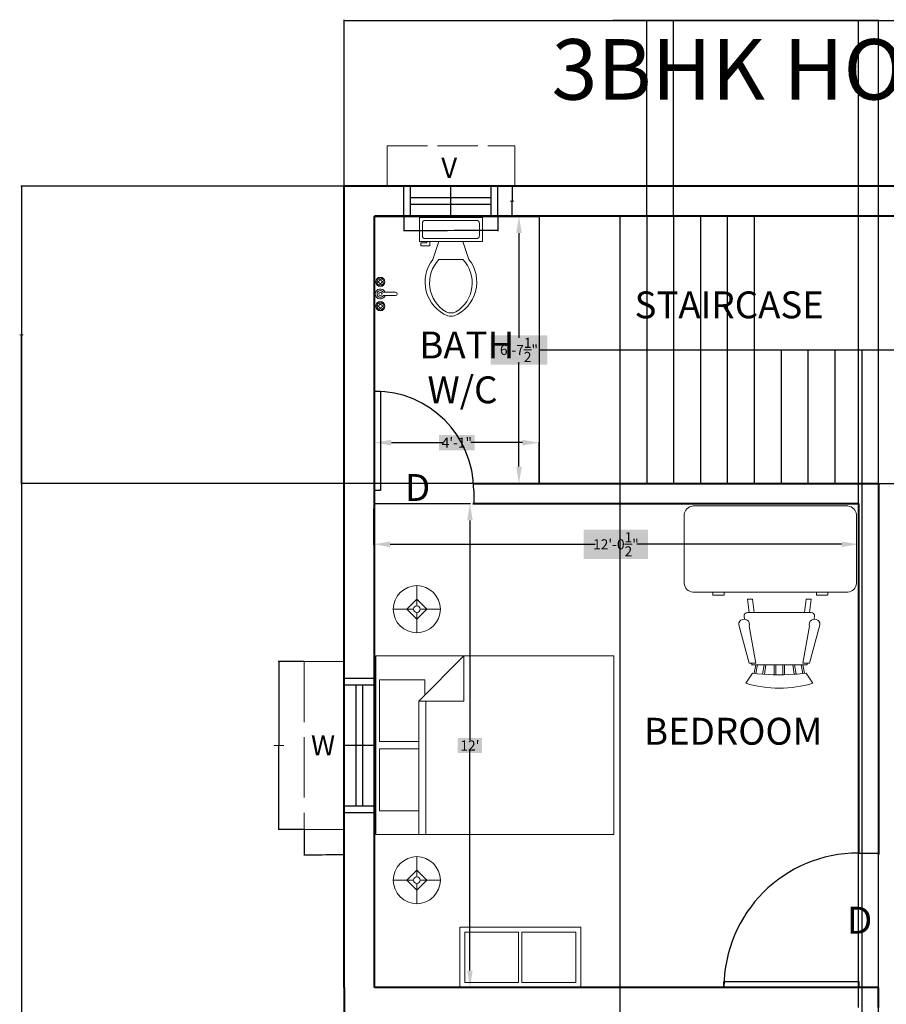
# Model space of a CAD drawing. Units: inches. Extents: x -301 to 715, y -607 to 364.
# Tile 104 of 141: x -301 to -43, y 67 to 360. Entities that reach past the tile are written whole.
import ezdxf

# ---------------------------------------------------------------- set-up
doc = ezdxf.new("R2010")
doc.units = ezdxf.units.IN
doc.header["$MEASUREMENT"] = 0
doc.linetypes.add('ACAD_ISO02W100', pattern=[15, 12, -3])
for name, color, linetype, lineweight in [('A-ANNO-DIMS', 2, 'Continuous', 18), ('A-ANNO-TEXT', 4, 'Continuous', 18), ('A-ANNO-TITL', 1, 'Continuous', 35), ('A-AREA-IDEN', 220, 'Continuous', 25), ('A-DOOR', 4, 'Continuous', 25), ('A-FLOR-CASE', 8, 'Continuous', 18), ('A-FLOR-FIXT', 9, 'Continuous', 18), ('A-FLOR-STRS', 2, 'Continuous', 25), ('A-FURN', 8, 'Continuous', 18), ('A-GLAZ', 2, 'Continuous', 25), ('A-GLAZ-OVHD', 2, 'ACAD_ISO02W100', 18), ('A-WALL', 3, 'Continuous', 40)]:
    doc.layers.add(name, color=color, linetype=linetype, lineweight=lineweight)
doc.styles.get("Standard").update_dxf_attribs({"font": 'arial.ttf'})
doc.dimstyles.get("Standard").update_dxf_attribs({"dimtxt": 0.18, "dimasz": 0.18, "dimexe": 0.18, "dimexo": 0.0625, "dimgap": 0.09, "dimtad": 0, "dimtih": 1, "dimtoh": 1, "dimdec": 1, "dimzin": 0, "dimdsep": 46, "dimlunit": 4, "dimtxsty": 'Standard', "dimcen": 0.09, "dimclrd": 3, "dimclre": 4, "dimclrt": 6, "dimadec": 0, "dimazin": 0, "dimtfac": 1, "dimtdec": 1, "dimtofl": 0, "dimtmove": 0, "dimatfit": 3, "dimfxl": 1, "dimtfill": 2, "dimtfillclr": 51, "dimtolj": 1, "dimtzin": 0, "dimarcsym": 0})

# ---------------------------------------------------------------- blocks, each defined once
blk = doc.blocks.new('*U4')
for p, q in [((0, 0), (0, -6)), ((40, 0), (40, -6))]:
    blk.add_line(p, q)
blk.add_lwpolyline([(0, 0), (0, 40), (1.75, 40), (1.75, 0)], close=True)
blk.add_arc((0, 0), 40, 0, 90)
blk = doc.blocks.new('Bed - Queen')
for p, q in [((0, -80.00003), (0, 0)), ((0, 0), (59.99999, 0)), ((59.99999, 0), (59.99999, -80.00003)), ((7.99999, -1.2), (28.79998, -1.2)), ((7.99999, -14.4), (7.99999, -1.2)), ((28.79998, -1.2), (28.79998, -14.4)), ((31.19999, -1.2), (51.99999, -1.2)), ((31.19999, -14.4), (31.19999, -1.2)), ((51.99999, -1.2), (51.99999, -16.4)), ((0, -14.4), (44.8, -14.4)), ((59.99999, -29.6), (44.8, -14.4)), ((44.8, -14.4), (44.8, -29.6)), ((51.99999, -16.4), (46.79936, -16.4)), ((44.8, -16.8), (0, -16.8)), ((44.8, -29.6), (59.99999, -29.6)), ((59.99999, -80.00003), (0, -80.00003))]:
    blk.add_line(p, q)
blk = doc.blocks.new('Lamp - Table')
for p, q in [((0, 7), (0, 1)), ((0, 3), (-3, 0)), ((3, 0), (0, 3)), ((-1, 0), (-7, 0)), ((-3, 0), (0, -3)), ((0, -3), (3, 0)), ((1, 0), (7, 0)), ((0, -1), (0, -7))]:
    blk.add_line(p, q)
for radius in [7, 1]:
    blk.add_circle((0, 0), radius)
blk = doc.blocks.new('Desk - 30 x 60 in.')
for p, q in [((-26.999995, 0), (26.999995, 0)), ((-29.999995, -27), (-29.999995, -3)), ((29.999995, -3), (29.999995, -27)), ((26.999995, -30), (-26.999995, -30)), ((-20.000005, -30), (-20.000005, -31)), ((-16.000005, -31), (-16.000005, -30)), ((15.999995, -31), (15.999995, -30)), ((19.999995, -30), (19.999995, -31)), ((-20.000005, -31), (-16.000005, -31)), ((19.999995, -31), (15.999995, -31))]:
    blk.add_line(p, q)
for centre, start, end in [((-26.499995, -3.5), 98.1301, 171.8699), ((26.499995, -3.5), 8.130102, 81.8699), ((-26.499995, -26.5), 188.1301, 261.8699), ((26.499995, -26.5), 278.1301, 351.8699)]:
    blk.add_arc(centre, 3.535534, start, end)
blk = doc.blocks.new('Chair - Rocking')
for p, q in [((-8, -4.5), (-10, -1.5)), ((8, -4.5), (10, -1.5)), ((-7.5, -4.5), (-7, -7)), ((-6.5, -7), (-7.02225, -4.43)), ((-4.5, -7), (-4.96674, -4.19951)), ((-4, -7), (-4.40532, -4.16272)), ((-1.5, -4.05012), (-1.5, -7)), ((-1, -7), (-1, -4.05012)), ((1, -7), (1, -4.04655)), ((1.5, -4.05012), (1.5, -7)), ((4, -7), (4.40187, -4.18694)), ((4.5, -7), (4.96761, -4.19437)), ((6.5, -7), (7, -4.4057)), ((7.5, -4.5), (7, -7)), ((-9, -7.5), (-12, -18.49999)), ((-7, -7.5), (-9, -7.5)), ((-9, -18.49999), (-7, -7.5)), ((-8.23428, -6.99939), (-8.3093, -7.47958)), ((-8.23041, -7), (8.23915, -7)), ((7, -7.5), (9, -7.5)), ((9, -18.49999), (7, -7.5)), ((8.31071, -7.48854), (8.23449, -7.00073)), ((9, -7.5), (12, -18.49999)), ((-10.36644, -20.64523), (-10.5, -21.49999)), ((-9, -22.49999), (-9.5, -26.49999)), ((0, -22.49999), (-9.5, -22.49999)), ((-8, -26.49999), (-7.5, -22.49999)), ((0, -22.49999), (9.5, -22.49999)), ((8, -26.49999), (7.5, -22.49999)), ((9, -22.49999), (9.5, -26.49999)), ((10.5, -21.49999), (10.3575, -20.58798)), ((-9.5, -26.49999), (-8, -26.49999)), ((9.5, -26.49999), (8, -26.49999))]:
    blk.add_line(p, q)
for centre, radius, start, end in [((0, -34.08333), 34.08333, 72.93847, 107.0615), ((0, -68.25004), 64.25, 93.92211, 97.15267), ((0, -68.25004), 64.25, 82.84733, 93.92211), ((-10.5, -18.99999), 1.58114, 161.5651, 18.43495), ((10.5, -18.99999), 1.58114, 161.5651, 18.43495), ((-9.5, -21.49999), 1, 180, 270), ((9.5, -21.49999), 1, 270, 0)]:
    blk.add_arc(centre, radius, start, end)
blk = doc.blocks.new('Wall Cabinet - 18 x 36 in front')
for p, q in [((17.5, -1.5), (17.5, -16.5)), ((18.5, -16.5), (18.5, -1.5))]:
    blk.add_line(p, q)
blk.add_lwpolyline([(0, -18), (0, 0), (36, 0), (36, -18)], close=True)
for points in [[(17.5, -16.5), (1.5, -16.5), (1.5, -1.5), (17.5, -1.5)], [(18.5, -1.5), (34.5, -1.5), (34.5, -16.5), (18.5, -16.5)]]:
    blk.add_lwpolyline(points)
blk = doc.blocks.new('*U2')
for p, q in [((0, 0), (0, -100)), ((750, 0), (750, -100))]:
    blk.add_line(p, q)
blk.add_lwpolyline([(0, 0), (0, 750), (43.75, 750), (43.75, 0)], close=True)
blk.add_arc((0, 0), 750, 0, 90)
blk = doc.blocks.new('Toilet - top')
for p, q in [((9.5, -6), (9.5, -2)), ((-10, -8.5), (-8, -8.5)), ((-10, -9.5), (-10, -8.5)), ((-7, -9.5), (-10, -9.5)), ((-8, -8.5), (-8, -8)), ((-7, -8), (-7, -9.5)), ((-4, -8), (-6, -14)), ((4, -8), (6, -14)), ((4, -14), (-4, -14))]:
    blk.add_line(p, q)
blk.add_lwpolyline([(10.5, -8), (10.5, 0), (-10.5, 0), (-10.5, -8)], close=True)
for points in [[(-9.5, -2), (-9.5, -6)], [(8.5, -1), (-8.5, -1)], [(-8.5, -7), (8.5, -7)]]:
    blk.add_lwpolyline(points)
for centre, radius, start, end in [((-8.62, -1.88), 0.884, 81.8699, 188.1301), ((8.62, -1.88), 0.884, 351.8699, 98.1301), ((-8.62, -6.12), 0.884, 171.8699, 278.1301), ((8.62, -6.12), 0.884, 261.8699, 8.1301), ((3.52, -21.58), 12.17, 141.4691, 247.9714), ((4.2, -21.82), 11.33, 136.3677, 238.9468), ((-3.52, -21.58), 12.17, 292.0284, 38.5307), ((-4.2, -21.82), 11.33, 301.053, 43.6321), ((0, -27.88), 4, 245.7318, 294.2682), ((0, -29), 4, 254.8605, 285.1395)]:
    blk.add_arc(centre, radius, start, end)
blk = doc.blocks.new('Faucet - Bathroom top')
for p, q in [((-4.107, 0.125), (-4.375, 0.125)), ((-3.75, 0.4788), (-3.75, 0.75)), ((-3.5, 0.482), (-3.5, 0.75)), ((-3.1461, 0.125), (-2.875, 0.125)), ((3.143, 0.125), (2.875, 0.125)), ((3.5, 0.4788), (3.5, 0.75)), ((3.75, 0.482), (3.75, 0.75)), ((4.1039, 0.125), (4.375, 0.125)), ((-4.1039, -0.125), (-4.375, -0.125)), ((-3.75, -0.4821), (-3.75, -0.75)), ((-3.5, -0.4789), (-3.5, -0.75)), ((-3.143, -0.125), (-2.875, -0.125)), ((-0.5, -0.8639), (-0.5, -4.5)), ((0.5, -4.5), (0.5, -0.8631)), ((3.1461, -0.125), (2.875, -0.125)), ((3.5, -0.4821), (3.5, -0.75)), ((3.75, -0.4789), (3.75, -0.75)), ((4.107, -0.125), (4.375, -0.125))]:
    blk.add_line(p, q)
for centre, radius in [((-3.625, 0), 1.375), ((-4.625, 0), 0.2795), ((-3.625, 0), 0.5), ((-3.625, 1), 0.2795), ((-2.625, 0), 0.2795), ((0, 0), 0.5), ((3.625, 0), 1.375), ((2.625, 0), 0.2795), ((3.625, 0), 0.5), ((3.625, 1), 0.2795), ((4.625, 0), 0.2795), ((-3.625, -1), 0.2795), ((3.625, -1), 0.2795)]:
    blk.add_circle(centre, radius)
for centre, radius, start, end in [((-3.625, 0), 1, 105.2407, 164.2093), ((-3.625, 0), 1, 16.44125, 74.07887), ((0, 0), 1.5, 289.6514, 250.3603), ((0, 0), 1, 300.3431, 239.7554), ((3.625, 0), 1, 106.12, 164.0884), ((3.625, 0), 1, 16.23422, 73.90469), ((-3.625, 0), 1, 196.2342, 253.9047), ((-3.625, 0), 1, 286.12, 344.0884), ((3.625, 0), 1, 196.4413, 254.0789), ((3.625, 0), 1, 285.2407, 344.2093), ((0, -4.5), 0.5, 180, 0)]:
    blk.add_arc(centre, radius, start, end)
blk = doc.blocks.new('*D52')
at = {"layer": 'A-ANNO-DIMS', "color": 0, "lineweight": -2, "transparency": 16777216}
for p, q in [((-195.6, 224.09), (-195.6, 234.01)), ((-190.6, 233.83), (-175.24, 233.83)), ((-151.6, 233.83), (-166.97, 233.83)), ((-146.6, 221.74), (-146.6, 234.01))]:
    blk.add_line(p, q, dxfattribs=at)
at = {"layer": 'A-ANNO-DIMS', "color": 0, "transparency": 16777216}
for points in [[(-190.6, 234.66), (-190.6, 232.99), (-195.6, 233.83)], [(-151.6, 234.66), (-151.6, 232.99), (-146.6, 233.83)]]:
    blk.add_solid(points, dxfattribs=at)
at = {"layer": 'Defpoints', "color": 0, "transparency": 16777216}
for p in [(-195.6, 233.83), (-195.6, 224.03), (-146.6, 221.68)]:
    blk.add_point(p, dxfattribs=at)
at = {"layer": 'A-ANNO-DIMS', "color": 0, "transparency": 16777216, "insert": (-171.1, 233.83), "char_height": 3, "attachment_point": 5, "bg_fill": 1, "box_fill_scale": 1.25, "bg_fill_color": 51, "bg_fill_transparency": 0}
blk.add_mtext('\\A1;4\'-1"', dxfattribs=at)
blk = doc.blocks.new('*D53')
at = {"layer": 'A-ANNO-DIMS', "color": 0, "lineweight": -2, "transparency": 16777216}
for p, q in [((-146.67, 301.18), (-152.79, 301.18)), ((-146.67, 221.68), (-152.79, 221.68))]:
    blk.add_line(p, q, dxfattribs=at)
at = {"layer": 'A-ANNO-DIMS', "color": 0, "lineweight": 30, "transparency": 16777216}
for p, q in [((-152.61, 296.18), (-152.61, 265.06)), ((-152.61, 226.68), (-152.61, 257.8))]:
    blk.add_line(p, q, dxfattribs=at)
at = {"layer": 'A-ANNO-DIMS', "color": 0, "transparency": 16777216}
for points in [[(-153.45, 296.18), (-151.78, 296.18), (-152.61, 301.18)], [(-153.45, 226.68), (-151.78, 226.68), (-152.61, 221.68)]]:
    blk.add_solid(points, dxfattribs=at)
at = {"layer": 'Defpoints', "color": 0, "transparency": 16777216}
for p in [(-146.6, 301.18), (-152.61, 221.68), (-146.6, 221.68)]:
    blk.add_point(p, dxfattribs=at)
at = {"layer": 'A-ANNO-DIMS', "color": 0, "transparency": 16777216, "insert": (-152.61, 261.43), "char_height": 3, "attachment_point": 5, "bg_fill": 1, "box_fill_scale": 1.25, "bg_fill_color": 51, "bg_fill_transparency": 0}
blk.add_mtext('\\A1;6\'-7{\\H1x;\\S1/2;}"', dxfattribs=at)
blk = doc.blocks.new('*D54')
at = {"layer": 'A-ANNO-DIMS', "color": 0, "lineweight": -2, "transparency": 16777216}
for p, q in [((-195.92, 214.14), (-195.92, 203.39)), ((-51.6, 215.62), (-51.6, 203.39)), ((-190.92, 203.57), (-129.96, 203.57)), ((-56.6, 203.57), (-117.57, 203.57))]:
    blk.add_line(p, q, dxfattribs=at)
at = {"layer": 'A-ANNO-DIMS', "color": 0, "transparency": 16777216}
for points in [[(-190.92, 204.4), (-190.92, 202.73), (-195.92, 203.57)], [(-56.6, 204.4), (-56.6, 202.73), (-51.6, 203.57)]]:
    blk.add_solid(points, dxfattribs=at)
at = {"layer": 'Defpoints', "color": 0, "transparency": 16777216}
for p in [(-195.92, 214.2), (-51.6, 215.68), (-195.92, 203.57)]:
    blk.add_point(p, dxfattribs=at)
at = {"layer": 'A-ANNO-DIMS', "color": 0, "transparency": 16777216, "insert": (-123.76, 203.57), "char_height": 3, "attachment_point": 5, "bg_fill": 1, "box_fill_scale": 1.25, "bg_fill_color": 51, "bg_fill_transparency": 0}
blk.add_mtext('\\A1;12\'-0{\\H1x;\\S1/2;}"', dxfattribs=at)
blk = doc.blocks.new('*D55')
at = {"layer": 'A-ANNO-DIMS', "color": 0, "lineweight": -2, "transparency": 16777216}
for p, q in [((-195.54, 215.68), (-167.03, 215.68)), ((-167.21, 210.68), (-167.21, 145.28)), ((-167.21, 76.68), (-167.21, 142.09)), ((-195.54, 71.68), (-167.03, 71.68))]:
    blk.add_line(p, q, dxfattribs=at)
at = {"layer": 'A-ANNO-DIMS', "color": 0, "transparency": 16777216}
for points in [[(-168.04, 210.68), (-166.38, 210.68), (-167.21, 215.68)], [(-168.04, 76.68), (-166.38, 76.68), (-167.21, 71.68)]]:
    blk.add_solid(points, dxfattribs=at)
at = {"layer": 'Defpoints', "color": 0, "transparency": 16777216}
for p in [(-195.6, 215.68), (-167.21, 215.68), (-195.6, 71.68)]:
    blk.add_point(p, dxfattribs=at)
at = {"layer": 'A-ANNO-DIMS', "color": 0, "transparency": 16777216, "insert": (-167.21, 143.68), "char_height": 3, "attachment_point": 5, "bg_fill": 1, "box_fill_scale": 1.25, "bg_fill_color": 51, "bg_fill_transparency": 0}
blk.add_mtext("\\A1;12'", dxfattribs=at)
blk = doc.blocks.new('WIN-36-PLAN')
for p, q in [((0, 0), (0, 9)), ((2, 0), (2, 9)), ((20, 0), (20, 9)), ((38, 0), (38, 9)), ((40, 0), (40, 9)), ((2, 5.5), (38, 5.5)), ((2, 3.5), (38, 3.5))]:
    blk.add_line(p, q)
blk = doc.blocks.new('VENT-24-PLAN')
for p, q in [((0, 0), (0, 9)), ((2, 0), (2, 9)), ((14, 0), (14, 9)), ((26, 0), (26, 9)), ((28, 0), (28, 9)), ((26, 5.5), (2, 5.5)), ((26, 3.5), (2, 3.5))]:
    blk.add_line(p, q)
blk = doc.blocks.new('WIN-SHADE-50')
at = {"ltscale": 1.5}
for p, q in [((0, 0), (0, 12)), ((50, 12), (0, 12)), ((50, 0), (50, 12)), ((5, 0), (0, 0)), ((45, 0), (50, 0))]:
    blk.add_line(p, q, dxfattribs=at)
blk = doc.blocks.new('VENT-SHADE-38')
for p, q in [((0, 0), (0, 12)), ((0, 12), (38, 12)), ((38, 0), (38, 12)), ((5, 0), (0, 0)), ((33, 0), (38, 0))]:
    blk.add_line(p, q)
blk = doc.blocks.new('*D98')
at = {"layer": 'A-ANNO-DIMS', "color": 4, "lineweight": -2, "transparency": 16777216}
for p, q in [((-216.67, 168.68), (-224.28, 168.68)), ((-216.67, 118.68), (-224.28, 118.68))]:
    blk.add_line(p, q, dxfattribs=at)
at = {"layer": 'A-ANNO-DIMS', "color": 3, "lineweight": -2, "transparency": 16777216}
for p, q in [((-224.1, 168.5), (-224.1, 143.87)), ((-224.1, 118.86), (-224.1, 143.5))]:
    blk.add_line(p, q, dxfattribs=at)
at = {"layer": 'A-ANNO-DIMS', "color": 3, "transparency": 16777216}
for points in [[(-224.13, 168.5), (-224.07, 168.5), (-224.1, 168.68)], [(-224.13, 118.86), (-224.07, 118.86), (-224.1, 118.68)]]:
    blk.add_solid(points, dxfattribs=at)
at = {"layer": 'Defpoints', "color": 0, "transparency": 16777216}
for p in [(-224.1, 168.68), (-216.6, 168.68), (-216.6, 118.68)]:
    blk.add_point(p, dxfattribs=at)
at = {"layer": 'A-ANNO-DIMS', "color": 6, "transparency": 16777216, "insert": (-224.1, 143.68), "char_height": 0.18, "attachment_point": 5, "bg_fill": 1, "box_fill_scale": 1.25, "bg_fill_color": 51, "bg_fill_transparency": 0}
blk.add_mtext('\\A1;WINDOW SHADE 4\'-2" TYP.', dxfattribs=at)
blk = doc.blocks.new('*D99')
at = {"layer": 'A-ANNO-DIMS', "color": 4, "lineweight": -2, "transparency": 16777216}
for p, q in [((-216.6, 118.62), (-216.6, 111)), ((-204.6, 118.62), (-204.6, 111))]:
    blk.add_line(p, q, dxfattribs=at)
at = {"layer": 'A-ANNO-DIMS', "color": 3, "lineweight": -2, "transparency": 16777216}
for p, q in [((-216.42, 111.18), (-211.23, 111.18)), ((-204.78, 111.18), (-209.97, 111.18))]:
    blk.add_line(p, q, dxfattribs=at)
at = {"layer": 'A-ANNO-DIMS', "color": 3, "transparency": 16777216}
for points in [[(-216.42, 111.21), (-216.42, 111.15), (-216.6, 111.18)], [(-204.78, 111.21), (-204.78, 111.15), (-204.6, 111.18)]]:
    blk.add_solid(points, dxfattribs=at)
at = {"layer": 'Defpoints', "color": 0, "transparency": 16777216}
for p in [(-216.6, 118.68), (-204.6, 118.68), (-216.6, 111.18)]:
    blk.add_point(p, dxfattribs=at)
at = {"layer": 'A-ANNO-DIMS', "color": 6, "transparency": 16777216, "insert": (-210.6, 111.18), "char_height": 0.18, "attachment_point": 5, "bg_fill": 1, "box_fill_scale": 1.25, "bg_fill_color": 51, "bg_fill_transparency": 0}
blk.add_mtext('\\A1;1\'-0" TYP.', dxfattribs=at)
blk = doc.blocks.new('*D100')
at = {"layer": 'A-ANNO-DIMS', "color": 4, "lineweight": -2, "transparency": 16777216}
for p, q in [((-186.87, 301.12), (-186.87, 296.8)), ((-158.87, 301.12), (-158.87, 296.8))]:
    blk.add_line(p, q, dxfattribs=at)
at = {"layer": 'A-ANNO-DIMS', "color": 3, "lineweight": -2, "transparency": 16777216}
for p, q in [((-186.69, 296.98), (-173.89, 296.98)), ((-159.05, 296.98), (-171.86, 296.98))]:
    blk.add_line(p, q, dxfattribs=at)
at = {"layer": 'A-ANNO-DIMS', "color": 3, "transparency": 16777216}
for points in [[(-186.69, 297.01), (-186.69, 296.95), (-186.87, 296.98)], [(-159.05, 297.01), (-159.05, 296.95), (-158.87, 296.98)]]:
    blk.add_solid(points, dxfattribs=at)
at = {"layer": 'Defpoints', "color": 0, "transparency": 16777216}
for p in [(-186.87, 301.18), (-158.87, 301.18), (-158.87, 296.98)]:
    blk.add_point(p, dxfattribs=at)
at = {"layer": 'A-ANNO-DIMS', "color": 6, "transparency": 16777216, "insert": (-172.87, 296.98), "char_height": 0.18, "attachment_point": 5, "bg_fill": 1, "box_fill_scale": 1.25, "bg_fill_color": 51, "bg_fill_transparency": 0}
blk.add_mtext('\\A1;VENT 2\'-4" TYP.', dxfattribs=at)
blk = doc.blocks.new('*D101')
at = {"layer": 'A-ANNO-DIMS', "color": 4, "lineweight": -2, "transparency": 16777216}
for p, q in [((-158.81, 310.18), (-154.49, 310.18)), ((-158.81, 301.18), (-154.49, 301.18))]:
    blk.add_line(p, q, dxfattribs=at)
at = {"layer": 'A-ANNO-DIMS', "color": 3, "lineweight": -2, "transparency": 16777216}
for p, q in [((-154.67, 310), (-154.67, 305.86)), ((-154.67, 301.36), (-154.67, 305.5))]:
    blk.add_line(p, q, dxfattribs=at)
at = {"layer": 'A-ANNO-DIMS', "color": 3, "transparency": 16777216}
for points in [[(-154.7, 310), (-154.64, 310), (-154.67, 310.18)], [(-154.7, 301.36), (-154.64, 301.36), (-154.67, 301.18)]]:
    blk.add_solid(points, dxfattribs=at)
at = {"layer": 'Defpoints', "color": 0, "transparency": 16777216}
for p in [(-158.87, 310.18), (-154.67, 310.18), (-158.87, 301.18)]:
    blk.add_point(p, dxfattribs=at)
at = {"layer": 'A-ANNO-DIMS', "color": 6, "transparency": 16777216, "insert": (-154.67, 305.68), "char_height": 0.18, "attachment_point": 5, "bg_fill": 1, "box_fill_scale": 1.25, "bg_fill_color": 51, "bg_fill_transparency": 0}
blk.add_mtext('\\A1;0\'-9" TYP.', dxfattribs=at)
blk = doc.blocks.new('*D144')
at = {"layer": 'A-ANNO-DIMS', "color": 4, "lineweight": -2, "transparency": 16777216}
for p, q in [((-204.6, 310.24), (-204.6, 359.61)), ((132.9, 310.24), (132.9, 359.61))]:
    blk.add_line(p, q, dxfattribs=at)
at = {"layer": 'A-ANNO-DIMS', "color": 3, "lineweight": -2, "transparency": 16777216}
for p, q in [((-204.42, 359.43), (-36.46, 359.43)), ((132.72, 359.43), (-35.24, 359.43))]:
    blk.add_line(p, q, dxfattribs=at)
at = {"layer": 'A-ANNO-DIMS', "color": 3, "transparency": 16777216}
for points in [[(-204.42, 359.46), (-204.42, 359.4), (-204.6, 359.43)], [(132.72, 359.46), (132.72, 359.4), (132.9, 359.43)]]:
    blk.add_solid(points, dxfattribs=at)
at = {"layer": 'Defpoints', "color": 0, "transparency": 16777216}
for p in [(132.9, 359.43), (-204.6, 310.18), (132.9, 310.18)]:
    blk.add_point(p, dxfattribs=at)
at = {"layer": 'A-ANNO-DIMS', "color": 6, "transparency": 16777216, "insert": (-35.85, 359.43), "char_height": 0.18, "attachment_point": 5, "bg_fill": 1, "box_fill_scale": 1.25, "bg_fill_color": 51, "bg_fill_transparency": 0}
blk.add_mtext('\\A1;28\'-1 1/2"', dxfattribs=at)
blk = doc.blocks.new('*D145')
at = {"layer": 'A-ANNO-DIMS', "color": 4, "lineweight": -2, "transparency": 16777216}
for p, q in [((-204.67, 310.18), (-300.87, 310.18)), ((-204.67, -223.82), (-300.87, -223.82))]:
    blk.add_line(p, q, dxfattribs=at)
at = {"layer": 'A-ANNO-DIMS', "color": 3, "lineweight": -2, "transparency": 16777216}
for p, q in [((-300.69, 310), (-300.69, 43.36)), ((-300.69, -223.64), (-300.69, 43))]:
    blk.add_line(p, q, dxfattribs=at)
at = {"layer": 'A-ANNO-DIMS', "color": 3, "transparency": 16777216}
for points in [[(-300.72, 310), (-300.66, 310), (-300.69, 310.18)], [(-300.72, -223.64), (-300.66, -223.64), (-300.69, -223.82)]]:
    blk.add_solid(points, dxfattribs=at)
at = {"layer": 'Defpoints', "color": 0, "transparency": 16777216}
for p in [(-300.69, 310.18), (-204.6, 310.18), (-204.6, -223.82)]:
    blk.add_point(p, dxfattribs=at)
at = {"layer": 'A-ANNO-DIMS', "color": 6, "transparency": 16777216, "insert": (-300.69, 43.18), "char_height": 0.18, "attachment_point": 5, "bg_fill": 1, "box_fill_scale": 1.25, "bg_fill_color": 51, "bg_fill_transparency": 0}
blk.add_mtext('\\A1;44\'-6"', dxfattribs=at)
blk = doc.blocks.new('*D150')
at = {"layer": 'A-ANNO-DIMS', "color": 4, "lineweight": -2, "transparency": 16777216}
for p, q in [((-51.6, 65.74), (-51.6, 359.61)), ((-45.6, 65.74), (-45.6, 359.61))]:
    blk.add_line(p, q, dxfattribs=at)
at = {"layer": 'A-ANNO-DIMS', "color": 3, "lineweight": -2, "transparency": 16777216}
for p, q in [((-51.42, 359.43), (-48.93, 359.43)), ((-45.78, 359.43), (-48.27, 359.43))]:
    blk.add_line(p, q, dxfattribs=at)
at = {"layer": 'A-ANNO-DIMS', "color": 3, "transparency": 16777216}
for points in [[(-51.42, 359.46), (-51.42, 359.4), (-51.6, 359.43)], [(-45.78, 359.46), (-45.78, 359.4), (-45.6, 359.43)]]:
    blk.add_solid(points, dxfattribs=at)
at = {"layer": 'Defpoints', "color": 0, "transparency": 16777216}
for p in [(-51.6, 359.43), (-51.6, 65.68), (-45.6, 65.68)]:
    blk.add_point(p, dxfattribs=at)
at = {"layer": 'A-ANNO-DIMS', "color": 6, "transparency": 16777216, "insert": (-48.6, 359.43), "char_height": 0.18, "attachment_point": 5, "bg_fill": 1, "box_fill_scale": 1.25, "bg_fill_color": 51, "bg_fill_transparency": 0}
blk.add_mtext('\\A1;0\'-6"', dxfattribs=at)
blk = doc.blocks.new('*D151')
at = {"layer": 'A-ANNO-DIMS', "color": 4, "lineweight": -2, "transparency": 16777216}
for p, q in [((-204.6, -223.76), (-204.6, 359.61)), ((-45.6, -214.76), (-45.6, 359.61))]:
    blk.add_line(p, q, dxfattribs=at)
at = {"layer": 'A-ANNO-DIMS', "color": 3, "lineweight": -2, "transparency": 16777216}
for p, q in [((-204.42, 359.43), (-125.49, 359.43)), ((-45.78, 359.43), (-124.71, 359.43))]:
    blk.add_line(p, q, dxfattribs=at)
at = {"layer": 'A-ANNO-DIMS', "color": 3, "transparency": 16777216}
for points in [[(-204.42, 359.46), (-204.42, 359.4), (-204.6, 359.43)], [(-45.78, 359.46), (-45.78, 359.4), (-45.6, 359.43)]]:
    blk.add_solid(points, dxfattribs=at)
at = {"layer": 'Defpoints', "color": 0, "transparency": 16777216}
for p in [(-45.6, 359.43), (-45.6, -214.82), (-204.6, -223.82)]:
    blk.add_point(p, dxfattribs=at)
at = {"layer": 'A-ANNO-DIMS', "color": 6, "transparency": 16777216, "insert": (-125.1, 359.43), "char_height": 0.18, "attachment_point": 5, "bg_fill": 1, "box_fill_scale": 1.25, "bg_fill_color": 51, "bg_fill_transparency": 0}
blk.add_mtext('\\A1;13\'-3"', dxfattribs=at)
blk = doc.blocks.new('*D155')
at = {"layer": 'A-ANNO-DIMS', "color": 4, "lineweight": -2, "transparency": 16777216}
for p, q in [((-204.67, 310.18), (-300.87, 310.18)), ((-146.67, 221.68), (-300.87, 221.68))]:
    blk.add_line(p, q, dxfattribs=at)
at = {"layer": 'A-ANNO-DIMS', "color": 3, "lineweight": -2, "transparency": 16777216}
for p, q in [((-300.69, 310), (-300.69, 266.12)), ((-300.69, 221.86), (-300.69, 265.75))]:
    blk.add_line(p, q, dxfattribs=at)
at = {"layer": 'A-ANNO-DIMS', "color": 3, "transparency": 16777216}
for points in [[(-300.72, 310), (-300.66, 310), (-300.69, 310.18)], [(-300.72, 221.86), (-300.66, 221.86), (-300.69, 221.68)]]:
    blk.add_solid(points, dxfattribs=at)
at = {"layer": 'Defpoints', "color": 0, "transparency": 16777216}
for p in [(-204.6, 310.18), (-300.69, 221.68), (-146.6, 221.68)]:
    blk.add_point(p, dxfattribs=at)
at = {"layer": 'A-ANNO-DIMS', "color": 6, "transparency": 16777216, "insert": (-300.69, 265.93), "char_height": 0.18, "attachment_point": 5, "bg_fill": 1, "box_fill_scale": 1.25, "bg_fill_color": 51, "bg_fill_transparency": 0}
blk.add_mtext('\\A1;7\'-4 1/2"', dxfattribs=at)
blk = doc.blocks.new('*D157')
at = {"layer": 'A-ANNO-DIMS', "color": 4, "lineweight": -2, "transparency": 16777216}
for p, q in [((-50.54, 261.43), (233.66, 261.43)), ((-50.54, 221.68), (233.66, 221.68))]:
    blk.add_line(p, q, dxfattribs=at)
at = {"layer": 'A-ANNO-DIMS', "color": 3, "lineweight": -2, "transparency": 16777216}
for p, q in [((233.48, 261.25), (233.48, 241.74)), ((233.48, 221.86), (233.48, 241.38))]:
    blk.add_line(p, q, dxfattribs=at)
at = {"layer": 'A-ANNO-DIMS', "color": 3, "transparency": 16777216}
for points in [[(233.45, 261.25), (233.51, 261.25), (233.48, 261.43)], [(233.45, 221.86), (233.51, 221.86), (233.48, 221.68)]]:
    blk.add_solid(points, dxfattribs=at)
at = {"layer": 'Defpoints', "color": 0, "transparency": 16777216}
for p in [(-50.6, 261.43), (233.48, 261.43), (-50.6, 221.68)]:
    blk.add_point(p, dxfattribs=at)
at = {"layer": 'A-ANNO-DIMS', "color": 6, "transparency": 16777216, "insert": (233.48, 241.56), "char_height": 0.18, "attachment_point": 5, "bg_fill": 1, "box_fill_scale": 1.25, "bg_fill_color": 51, "bg_fill_transparency": 0}
blk.add_mtext('\\A1;3\'-4"', dxfattribs=at)
blk = doc.blocks.new('*D158')
at = {"layer": 'A-ANNO-DIMS', "color": 4, "lineweight": -2, "transparency": 16777216}
for p, q in [((-122.6, 221.62), (-122.6, -296.87)), ((-50.6, 221.62), (-50.6, -296.87))]:
    blk.add_line(p, q, dxfattribs=at)
at = {"layer": 'A-ANNO-DIMS', "color": 3, "lineweight": -2, "transparency": 16777216}
for p, q in [((-122.42, -296.69), (-86.93, -296.69)), ((-50.78, -296.69), (-86.27, -296.69))]:
    blk.add_line(p, q, dxfattribs=at)
at = {"layer": 'A-ANNO-DIMS', "color": 3, "transparency": 16777216}
for points in [[(-122.42, -296.66), (-122.42, -296.72), (-122.6, -296.69)], [(-50.78, -296.66), (-50.78, -296.72), (-50.6, -296.69)]]:
    blk.add_solid(points, dxfattribs=at)
at = {"layer": 'Defpoints', "color": 0, "transparency": 16777216}
for p in [(-122.6, 221.68), (-50.6, 221.68), (-50.6, -296.69)]:
    blk.add_point(p, dxfattribs=at)
at = {"layer": 'A-ANNO-DIMS', "color": 6, "transparency": 16777216, "insert": (-86.6, -296.69), "char_height": 0.18, "attachment_point": 5, "bg_fill": 1, "box_fill_scale": 1.25, "bg_fill_color": 51, "bg_fill_transparency": 0}
blk.add_mtext('\\A1;6\'-0"', dxfattribs=at)
blk = doc.blocks.new('*D159')
at = {"layer": 'A-ANNO-DIMS', "color": 4, "lineweight": -2, "transparency": 16777216}
for p, q in [((-114.6, 301.24), (-114.6, 359.61)), ((-106.6, 301.24), (-106.6, 359.61))]:
    blk.add_line(p, q, dxfattribs=at)
at = {"layer": 'A-ANNO-DIMS', "color": 3, "lineweight": -2, "transparency": 16777216}
for p, q in [((-114.42, 359.43), (-110.93, 359.43)), ((-106.78, 359.43), (-110.27, 359.43))]:
    blk.add_line(p, q, dxfattribs=at)
at = {"layer": 'A-ANNO-DIMS', "color": 3, "transparency": 16777216}
for points in [[(-114.42, 359.46), (-114.42, 359.4), (-114.6, 359.43)], [(-106.78, 359.46), (-106.78, 359.4), (-106.6, 359.43)]]:
    blk.add_solid(points, dxfattribs=at)
at = {"layer": 'Defpoints', "color": 0, "transparency": 16777216}
for p in [(-106.6, 359.43), (-114.6, 301.18), (-106.6, 301.18)]:
    blk.add_point(p, dxfattribs=at)
at = {"layer": 'A-ANNO-DIMS', "color": 6, "transparency": 16777216, "insert": (-110.6, 359.43), "char_height": 0.18, "attachment_point": 5, "bg_fill": 1, "box_fill_scale": 1.25, "bg_fill_color": 51, "bg_fill_transparency": 0}
blk.add_mtext('\\A1;0\'-8"', dxfattribs=at)

msp = doc.modelspace()

# ---------------------------------------------------------------- linework, layer by layer
at = {"layer": 'A-FLOR-STRS'}
for p, q in [((-146.6, 301.18), (-146.6, 221.68)), ((-122.6, 301.18), (-122.6, 221.68)), ((-114.6, 301.18), (-114.6, 221.68)), ((-106.6, 301.18), (-106.6, 221.68)), ((-98.6, 301.18), (-98.6, 221.68)), ((-90.6, 301.18), (-90.6, 221.68)), ((-82.6, 301.18), (-82.6, 221.68)), ((-146.6, 261.43), (-50.6, 261.43)), ((-74.6, 261.43), (-74.6, 221.68)), ((-66.6, 261.43), (-66.6, 221.68)), ((-58.6, 261.43), (-58.6, 221.68)), ((-50.6, 261.43), (-50.6, 221.68))]:
    msp.add_line(p, q, dxfattribs=at)
at = {"layer": 'A-GLAZ'}
msp.add_line((-172.87, 301.18), (-172.87, 309.82), dxfattribs=at)
at = {"layer": 'A-WALL'}
for p, q in [((132.9, 310.18), (-204.6, 310.18)), ((-204.6, 71.68), (-204.6, 310.18)), ((-195.6, 301.18), (-146.6, 301.18)), ((-195.6, 215.68), (-195.6, 301.18)), ((9.9, 301.18), (-195.6, 301.18)), ((-166.15, 221.68), (-45.6, 221.68)), ((-45.6, 221.68), (-45.6, 193.18)), ((-195.6, 71.68), (-195.6, 215.68)), ((-166.34, 215.68), (-51.6, 215.68)), ((-51.6, 215.68), (-51.6, 111.68)), ((-45.6, 193.18), (-45.6, 111.23)), ((-51.6, 73.43), (-51.6, 71.68)), ((-204.6, 71.68), (-204.6, -67.32)), ((-45.6, 71.68), (-195.6, 71.68)), ((-45.6, 65.68), (-45.6, 71.68))]:
    msp.add_line(p, q, dxfattribs=at)

# ---------------------------------------------------------------- block references
at = {"layer": 'A-DOOR', "xscale": 0.0393700787401575, "yscale": 0.0393700787401575, "zscale": 0.0393700787401575}
msp.add_blockref('*U2', (-195.6, 219.62), dxfattribs=at)
at = {"layer": 'A-DOOR', "rotation": 90}
msp.add_blockref('*U4', (-51.6, 71.68), dxfattribs=at)
at = {"layer": 'A-FLOR-CASE'}
msp.add_blockref('Wall Cabinet - 18 x 36 in front', (-170.22, 89.67), dxfattribs=at)
at = {"layer": 'A-FLOR-FIXT', "xscale": 0.8906747211908207, "yscale": 0.8906747211908207, "zscale": 0.8906747211908207}
msp.add_blockref('Toilet - top', (-172.87, 300.82), dxfattribs=at)
at = {"layer": 'A-FLOR-FIXT', "rotation": 90}
msp.add_blockref('Faucet - Bathroom top', (-193.87, 278.07), dxfattribs=at)
at = {"layer": 'A-FURN', "xscale": 0.8558048107780498, "yscale": 0.8558048107780498, "zscale": 0.8558048107780498}
msp.add_blockref('Desk - 30 x 60 in.', (-77.8, 214.98), dxfattribs=at)
at = {"layer": 'A-FURN'}
for p in [(-183.02, 184.26), (-183.02, 103.61)]:
    msp.add_blockref('Lamp - Table', p, dxfattribs=at)
at = {"layer": 'A-FURN', "rotation": 180}
msp.add_blockref('Chair - Rocking', (-75.12, 160.73), dxfattribs=at)
at = {"layer": 'A-FURN', "xscale": 0.8856750462000775, "yscale": 0.8856750462000775, "zscale": 0.8856750462000775, "rotation": 90}
msp.add_blockref('Bed - Queen', (-195.21, 117.21), dxfattribs=at)
at = {"layer": 'A-GLAZ'}
msp.add_blockref('VENT-24-PLAN', (-186.87, 301.18), dxfattribs=at)
at = {"layer": 'A-GLAZ', "rotation": 90.00000000000036}
msp.add_blockref('WIN-36-PLAN', (-195.6, 123.68), dxfattribs=at)
at = {"layer": 'A-GLAZ-OVHD'}
msp.add_blockref('VENT-SHADE-38', (-191.87, 310.18), dxfattribs=at)
at = {"layer": 'A-GLAZ-OVHD', "rotation": 90.00000000000011}
msp.add_blockref('WIN-SHADE-50', (-204.6, 118.68), dxfattribs=at)

# ---------------------------------------------------------------- texts
at = {"layer": 'A-ANNO-TEXT'}
for s, height, p in [('V', 6, (-175.74, 312.61)), ('D', 8, (-186.53, 216.47)), ('W', 6, (-214.52, 140.74)), ('D', 8, (-54.97, 87.7))]:
    msp.add_text(s, height=height, dxfattribs=at).set_placement(p)
at = {"layer": 'A-ANNO-TITL'}
msp.add_text('3BHK HOME PLAN', height=18, dxfattribs=at).set_placement((-142.9, 335.91))
at = {"layer": 'A-AREA-IDEN', "char_height": 8, "attachment_point": 1}
for s, insert in [('STAIRCASE', (-118.21, 278.83)), ('BATH\\P W/C', (-182.29, 266.88)), ('BEDROOM', (-115.39, 151.93))]:
    msp.add_mtext_dynamic_manual_height_columns(s, width=73.06, gutter_width=1, heights=[0], dxfattribs=dict(at, insert=insert))

# ---------------------------------------------------------------- dimensions: what is measured, and where the dimension line sits
at = {"layer": 'A-ANNO-DIMS'}
for base, p1, p2, override, picture, middle in [((132.9, 359.43), (-204.6, 310.18), (132.9, 310.18), {"dimdec": 1, "dimlfac": 1, "dimrnd": 0, "dimzin": 1, "dimdsep": 46, "dimlunit": 4, "dimfrac": 2}, '*D144', (-35.85, 359.43)), ((-45.6, 359.43), (-204.6, -223.82), (-45.6, -214.82), {"dimdec": 1, "dimlfac": 1, "dimrnd": 0, "dimzin": 1, "dimdsep": 46, "dimlunit": 4, "dimfrac": 2}, '*D151', (-125.1, 359.43)), ((-106.6, 359.43), (-114.6, 301.18), (-106.6, 301.18), {"dimdec": 1, "dimlfac": 1, "dimrnd": 0, "dimzin": 1, "dimdsep": 46, "dimlunit": 4, "dimfrac": 2}, '*D159', (-110.6, 359.43)), ((-51.6, 359.43), (-45.6, 65.68), (-51.6, 65.68), {"dimdec": 1, "dimlfac": 1, "dimrnd": 0, "dimzin": 1, "dimdsep": 46, "dimlunit": 4, "dimfrac": 2}, '*D150', (-48.6, 359.43)), ((-195.6, 233.83), (-146.6, 221.68), (-195.6, 224.03), {"dimtxt": 3, "dimasz": 5, "dimclrd": 0, "dimclre": 0, "dimclrt": 0}, '*D52', (-171.1, 233.83)), ((-50.6, -296.69), (-122.6, 221.68), (-50.6, 221.68), {"dimdec": 1, "dimlfac": 1, "dimrnd": 0, "dimzin": 1, "dimdsep": 46, "dimlunit": 4, "dimfrac": 2}, '*D158', (-86.6, -296.69)), ((-195.92, 203.57), (-51.6, 215.68), (-195.92, 214.2), {"dimtxt": 3, "dimasz": 5, "dimclrd": 0, "dimclre": 0, "dimclrt": 0}, '*D54', (-123.76, 203.57))]:
    dim = msp.add_linear_dim(base=base, p1=p1, p2=p2, dimstyle='Standard', override=override, dxfattribs=at)
    dim.commit()
    dim.dimension.update_dxf_attribs({"geometry": picture, "text_midpoint": middle})
for base, p1, p2, override, picture, middle in [((-300.69, 221.68), (-204.6, 310.18), (-146.6, 221.68), {"dimdec": 1, "dimlfac": 1, "dimrnd": 0, "dimzin": 1, "dimdsep": 46, "dimlunit": 4, "dimfrac": 2}, '*D155', (-300.69, 265.93)), ((-300.69, 310.18), (-204.6, -223.82), (-204.6, 310.18), {"dimdec": 1, "dimlfac": 1, "dimrnd": 0, "dimzin": 1, "dimdsep": 46, "dimlunit": 4, "dimfrac": 2}, '*D145', (-300.69, 43.18)), ((-152.61, 221.68), (-146.6, 301.18), (-146.6, 221.68), {"dimtxt": 3, "dimasz": 5, "dimclrd": 0, "dimclre": 0, "dimclrt": 0, "dimlwd": 30}, '*D53', (-152.61, 261.43)), ((233.479242, 261.43233), (-50.603288, 221.68233), (-50.603288, 261.43233), {"dimdec": 1, "dimlfac": 1, "dimrnd": 0, "dimzin": 1, "dimdsep": 46, "dimlunit": 4, "dimfrac": 2}, '*D157', (233.479242, 241.55733)), ((-167.21, 215.68), (-195.6, 71.68), (-195.6, 215.68), {"dimtxt": 3, "dimasz": 5, "dimclrd": 0, "dimclre": 0, "dimclrt": 0}, '*D55', (-167.21, 143.68))]:
    dim = msp.add_linear_dim(base=base, p1=p1, p2=p2, angle=90, dimstyle='Standard', override=override, dxfattribs=at)
    dim.commit()
    dim.dimension.update_dxf_attribs({"geometry": picture, "text_midpoint": middle})
for base, p1, p2, angle, text, picture, middle in [((-154.67, 310.18), (-158.87, 301.18), (-158.87, 310.18), 90, '<> TYP.', '*D101', (-154.67, 305.68)), ((-224.1, 168.68), (-216.6, 118.68), (-216.6, 168.68), 90, 'WINDOW SHADE <> TYP.', '*D98', (-224.1, 143.68)), ((-216.6, 111.18), (-204.6, 118.68), (-216.6, 118.68), 180, '<> TYP.', '*D99', (-210.6, 111.18))]:
    dim = msp.add_linear_dim(base=base, p1=p1, p2=p2, angle=angle, text=text, dimstyle='Standard', override={"dimdec": 1, "dimlfac": 1, "dimrnd": 0, "dimzin": 1, "dimdsep": 46, "dimlunit": 4, "dimfrac": 2}, dxfattribs=at)
    dim.commit()
    dim.dimension.update_dxf_attribs({"geometry": picture, "text_midpoint": middle})
dim = msp.add_linear_dim(base=(-158.87, 296.98), p1=(-186.87, 301.18), p2=(-158.87, 301.18), text='VENT <> TYP.', dimstyle='Standard', override={"dimdec": 1, "dimlfac": 1, "dimrnd": 0, "dimzin": 1, "dimdsep": 46, "dimlunit": 4, "dimfrac": 2}, dxfattribs=at)
dim.commit()
dim.dimension.update_dxf_attribs({"geometry": '*D100', "text_midpoint": (-172.87, 296.98)})

doc.saveas('drawing.dxf')
